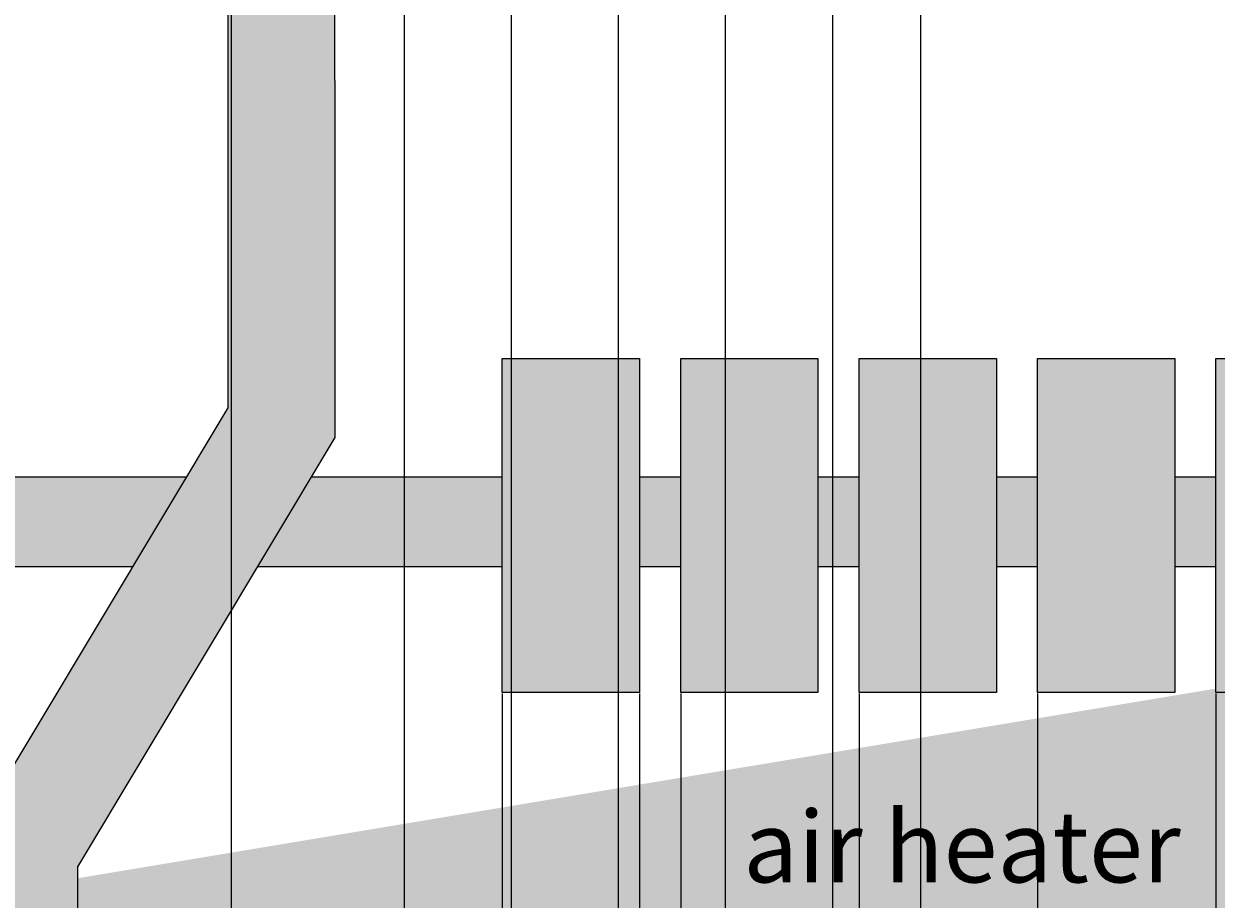
# Model space of a CAD drawing. Units: millimetres. Extents: x -22994 to 29398, y -19990 to 20176.
# Tile 109 of 135: x 99 to 166, y 124 to 174. Entities that reach past the tile are written whole.
import ezdxf

# ---------------------------------------------------------------- set-up
doc = ezdxf.new("R2010")
doc.units = ezdxf.units.MM
doc.header["$MEASUREMENT"] = 0
for name, color, linetype, lineweight in [('M-ANNO-TEXT', 7, 'Continuous', 25), ('M-DIMS', 2, 'Continuous', 18), ('M-EQPM', 7, 'Continuous', 25), ('M-EQPM-PATT', 7, 'Continuous', 18)]:
    doc.layers.add(name, color=color, linetype=linetype, lineweight=lineweight)
doc.styles.get("Standard").update_dxf_attribs({"font": 'arial.ttf'})
doc.dimstyles.get("Standard").update_dxf_attribs({"dimtxt": 0.18, "dimasz": 10000, "dimexe": 0.18, "dimexo": 0.0625, "dimgap": 0.09, "dimtad": 0, "dimtih": 1, "dimtoh": 1, "dimdec": 0, "dimzin": 0, "dimdsep": 46, "dimtxsty": 'Standard', "dimcen": 0.09, "dimadec": 0, "dimazin": 0, "dimtfac": 1, "dimtdec": 0, "dimtofl": 0, "dimtmove": 0, "dimatfit": 3, "dimfxl": 1, "dimtolj": 1, "dimtzin": 0, "dimlwd": 30, "dimarcsym": 0})

# ---------------------------------------------------------------- blocks, each defined once
blk = doc.blocks.new('*D2')
at = {"layer": 'Defpoints', "color": 0, "transparency": 16777216}
for p in [(6.677, 10.271), (290.852, 10.271), (290.852, -5.079)]:
    blk.add_point(p, dxfattribs=at)
at = {"layer": 'M-DIMS', "color": 0, "lineweight": -2, "transparency": 16777216}
for p, q in [((6.677, 10.209), (6.677, -5.259)), ((290.852, 10.209), (290.852, -5.259))]:
    blk.add_line(p, q, dxfattribs=at)
at = {"layer": 'M-DIMS', "color": 0, "lineweight": 30, "transparency": 16777216}
for p, q in [((-9993.323, -5.079), (-19993.323, -5.079)), ((10290.852, -5.079), (20290.852, -5.079))]:
    blk.add_line(p, q, dxfattribs=at)
at = {"layer": 'M-DIMS', "color": 0, "transparency": 16777216}
for points in [[(-9993.323, 1661.588), (-9993.323, -1671.745), (6.677, -5.079)], [(10290.852, 1661.588), (10290.852, -1671.745), (290.852, -5.079)]]:
    blk.add_solid(points, dxfattribs=at)
at = {"layer": 'M-DIMS', "color": 0, "transparency": 16777216, "insert": (148.765, -5.079), "char_height": 0.18, "attachment_point": 5}
blk.add_mtext('\\A1;284.2', dxfattribs=at)
blk = doc.blocks.new('*D3')
at = {"layer": 'Defpoints', "color": 0, "transparency": 16777216}
for p in [(110.265, 204.165), (110.265, 176.366), (95.833, 127.967)]:
    blk.add_point(p, dxfattribs=at)
at = {"layer": 'M-DIMS', "color": 0, "lineweight": 30, "transparency": 16777216}
for p, q in [((-9904.167, 204.165), (-19904.167, 204.165)), ((10110.265, 204.165), (20110.265, 204.165))]:
    blk.add_line(p, q, dxfattribs=at)
at = {"layer": 'M-DIMS', "color": 0, "lineweight": -2, "transparency": 16777216}
for p, q in [((95.833, 128.03), (95.833, 204.345)), ((110.265, 176.429), (110.265, 204.345))]:
    blk.add_line(p, q, dxfattribs=at)
at = {"layer": 'M-DIMS', "color": 0, "transparency": 16777216}
for points in [[(-9904.167, 1870.832), (-9904.167, -1462.501), (95.833, 204.165)], [(10110.265, 1870.832), (10110.265, -1462.501), (110.265, 204.165)]]:
    blk.add_solid(points, dxfattribs=at)
at = {"layer": 'M-DIMS', "color": 0, "transparency": 16777216, "insert": (103.049, 204.165), "char_height": 0.18, "attachment_point": 5}
blk.add_mtext('\\A1;14.432', dxfattribs=at)
blk = doc.blocks.new('*D4')
at = {"layer": 'Defpoints', "color": 0, "transparency": 16777216}
for p in [(116.265, 204.165), (110.265, 176.366), (116.265, 176.366)]:
    blk.add_point(p, dxfattribs=at)
at = {"layer": 'M-DIMS', "color": 0, "lineweight": 30, "transparency": 16777216}
for p, q in [((-9889.735, 204.165), (-19889.735, 204.165)), ((10116.265, 204.165), (20116.265, 204.165))]:
    blk.add_line(p, q, dxfattribs=at)
at = {"layer": 'M-DIMS', "color": 0, "lineweight": -2, "transparency": 16777216}
for p, q in [((110.265, 176.429), (110.265, 204.345)), ((116.265, 176.429), (116.265, 204.345))]:
    blk.add_line(p, q, dxfattribs=at)
at = {"layer": 'M-DIMS', "color": 0, "transparency": 16777216}
for points in [[(-9889.735, 1870.832), (-9889.735, -1462.501), (110.265, 204.165)], [(10116.265, 1870.832), (10116.265, -1462.501), (116.265, 204.165)]]:
    blk.add_solid(points, dxfattribs=at)
at = {"layer": 'M-DIMS', "color": 0, "transparency": 16777216, "insert": (113.265, 204.165), "char_height": 0.18, "attachment_point": 5}
blk.add_mtext('\\A1;6', dxfattribs=at)
blk = doc.blocks.new('*D5')
at = {"layer": 'Defpoints', "color": 0, "transparency": 16777216}
for p in [(181.265, 204.165), (116.265, 176.366), (181.265, 176.366)]:
    blk.add_point(p, dxfattribs=at)
at = {"layer": 'M-DIMS', "color": 0, "lineweight": 30, "transparency": 16777216}
for p, q in [((-9883.735, 204.165), (-19883.735, 204.165)), ((10181.265, 204.165), (20181.265, 204.165))]:
    blk.add_line(p, q, dxfattribs=at)
at = {"layer": 'M-DIMS', "color": 0, "lineweight": -2, "transparency": 16777216}
for p, q in [((116.265, 176.429), (116.265, 204.345)), ((181.265, 176.429), (181.265, 204.345))]:
    blk.add_line(p, q, dxfattribs=at)
at = {"layer": 'M-DIMS', "color": 0, "transparency": 16777216}
for points in [[(-9883.735, 1870.832), (-9883.735, -1462.501), (116.265, 204.165)], [(10181.265, 1870.832), (10181.265, -1462.501), (181.265, 204.165)]]:
    blk.add_solid(points, dxfattribs=at)
at = {"layer": 'M-DIMS', "color": 0, "transparency": 16777216, "insert": (148.765, 204.165), "char_height": 0.18, "attachment_point": 5}
blk.add_mtext('\\A1;65', dxfattribs=at)
blk = doc.blocks.new('*D6')
at = {"layer": 'Defpoints', "color": 0, "transparency": 16777216}
for p in [(187.265, 204.165), (181.265, 176.366), (187.265, 176.366)]:
    blk.add_point(p, dxfattribs=at)
at = {"layer": 'M-DIMS', "color": 0, "lineweight": 30, "transparency": 16777216}
for p, q in [((-9818.735, 204.165), (-19818.735, 204.165)), ((10187.265, 204.165), (20187.265, 204.165))]:
    blk.add_line(p, q, dxfattribs=at)
at = {"layer": 'M-DIMS', "color": 0, "lineweight": -2, "transparency": 16777216}
for p, q in [((181.265, 176.429), (181.265, 204.345)), ((187.265, 176.429), (187.265, 204.345))]:
    blk.add_line(p, q, dxfattribs=at)
at = {"layer": 'M-DIMS', "color": 0, "transparency": 16777216}
for points in [[(-9818.735, 1870.832), (-9818.735, -1462.501), (181.265, 204.165)], [(10187.265, 1870.832), (10187.265, -1462.501), (187.265, 204.165)]]:
    blk.add_solid(points, dxfattribs=at)
at = {"layer": 'M-DIMS', "color": 0, "transparency": 16777216, "insert": (184.265, 204.165), "char_height": 0.18, "attachment_point": 5}
blk.add_mtext('\\A1;6', dxfattribs=at)
blk = doc.blocks.new('*D7')
at = {"layer": 'Defpoints', "color": 0, "transparency": 16777216}
for p in [(201.697, 204.165), (187.265, 176.366), (201.697, 127.967)]:
    blk.add_point(p, dxfattribs=at)
at = {"layer": 'M-DIMS', "color": 0, "lineweight": 30, "transparency": 16777216}
for p, q in [((-9812.735, 204.165), (-19812.735, 204.165)), ((10201.697, 204.165), (20201.697, 204.165))]:
    blk.add_line(p, q, dxfattribs=at)
at = {"layer": 'M-DIMS', "color": 0, "lineweight": -2, "transparency": 16777216}
for p, q in [((187.265, 176.429), (187.265, 204.345)), ((201.697, 128.03), (201.697, 204.345))]:
    blk.add_line(p, q, dxfattribs=at)
at = {"layer": 'M-DIMS', "color": 0, "transparency": 16777216}
for points in [[(-9812.735, 1870.832), (-9812.735, -1462.501), (187.265, 204.165)], [(10201.697, 1870.832), (10201.697, -1462.501), (201.697, 204.165)]]:
    blk.add_solid(points, dxfattribs=at)
at = {"layer": 'M-DIMS', "color": 0, "transparency": 16777216, "insert": (194.481, 204.165), "char_height": 0.18, "attachment_point": 5}
blk.add_mtext('\\A1;14.432', dxfattribs=at)
blk = doc.blocks.new('*D8')
at = {"layer": 'Defpoints', "color": 0, "transparency": 16777216}
for p in [(227.648, 204.165), (227.648, 146.73), (201.697, 127.967)]:
    blk.add_point(p, dxfattribs=at)
at = {"layer": 'M-DIMS', "color": 0, "lineweight": 30, "transparency": 16777216}
for p, q in [((-9798.303, 204.165), (-19798.303, 204.165)), ((10227.648, 204.165), (20227.648, 204.165))]:
    blk.add_line(p, q, dxfattribs=at)
at = {"layer": 'M-DIMS', "color": 0, "lineweight": -2, "transparency": 16777216}
for p, q in [((201.697, 128.03), (201.697, 204.345)), ((227.648, 146.792), (227.648, 204.345))]:
    blk.add_line(p, q, dxfattribs=at)
at = {"layer": 'M-DIMS', "color": 0, "transparency": 16777216}
for points in [[(-9798.303, 1870.832), (-9798.303, -1462.501), (201.697, 204.165)], [(10227.648, 1870.832), (10227.648, -1462.501), (227.648, 204.165)]]:
    blk.add_solid(points, dxfattribs=at)
at = {"layer": 'M-DIMS', "color": 0, "transparency": 16777216, "insert": (214.673, 204.165), "char_height": 0.18, "attachment_point": 5}
blk.add_mtext('\\A1;25.95', dxfattribs=at)
blk = doc.blocks.new('*D9')
at = {"layer": 'Defpoints', "color": 0, "transparency": 16777216}
for p in [(187.265, 176.366), (306.202, 176.366), (290.852, 10.271)]:
    blk.add_point(p, dxfattribs=at)
at = {"layer": 'M-DIMS', "color": 0, "lineweight": 30, "transparency": 16777216}
for p, q in [((306.202, 10176.366), (306.202, 20176.366)), ((306.202, -9989.729), (306.202, -19989.729))]:
    blk.add_line(p, q, dxfattribs=at)
at = {"layer": 'M-DIMS', "color": 0, "lineweight": -2, "transparency": 16777216}
for p, q in [((187.327, 176.366), (306.382, 176.366)), ((290.915, 10.271), (306.382, 10.271))]:
    blk.add_line(p, q, dxfattribs=at)
at = {"layer": 'M-DIMS', "color": 0, "transparency": 16777216}
for points in [[(-1360.465, 10176.366), (1972.869, 10176.366), (306.202, 176.366)], [(-1360.465, -9989.729), (1972.869, -9989.729), (306.202, 10.271)]]:
    blk.add_solid(points, dxfattribs=at)
at = {"layer": 'M-DIMS', "color": 0, "transparency": 16777216, "insert": (306.202, 93.319), "char_height": 0.18, "attachment_point": 5}
blk.add_mtext('\\A1;166.1', dxfattribs=at)
blk = doc.blocks.new('*D10')
at = {"layer": 'Defpoints', "color": 0, "transparency": 16777216}
for p in [(125.65, 136.071), (133.346, 136.071), (133.346, -5.079)]:
    blk.add_point(p, dxfattribs=at)
at = {"layer": 'M-DIMS', "color": 0, "lineweight": -2, "transparency": 16777216}
for p, q in [((125.65, 136.009), (125.65, -5.259)), ((133.346, 136.009), (133.346, -5.259))]:
    blk.add_line(p, q, dxfattribs=at)
at = {"layer": 'M-DIMS', "color": 0, "lineweight": 30, "transparency": 16777216}
for p, q in [((-9874.35, -5.079), (-19874.35, -5.079)), ((10133.346, -5.079), (20133.346, -5.079))]:
    blk.add_line(p, q, dxfattribs=at)
at = {"layer": 'M-DIMS', "color": 0, "transparency": 16777216}
for points in [[(-9874.35, 1661.588), (-9874.35, -1671.745), (125.65, -5.079)], [(10133.346, 1661.588), (10133.346, -1671.745), (133.346, -5.079)]]:
    blk.add_solid(points, dxfattribs=at)
at = {"layer": 'M-DIMS', "color": 0, "transparency": 16777216, "insert": (129.498, -5.079), "char_height": 0.18, "attachment_point": 5}
blk.add_mtext('\\A1;7.696', dxfattribs=at)
blk = doc.blocks.new('*D11')
at = {"layer": 'Defpoints', "color": 0, "transparency": 16777216}
for p in [(133.346, 136.071), (135.65, 136.071), (135.65, -5.079)]:
    blk.add_point(p, dxfattribs=at)
at = {"layer": 'M-DIMS', "color": 0, "lineweight": -2, "transparency": 16777216}
for p, q in [((133.346, 136.009), (133.346, -5.259)), ((135.65, 136.009), (135.65, -5.259))]:
    blk.add_line(p, q, dxfattribs=at)
at = {"layer": 'M-DIMS', "color": 0, "lineweight": 30, "transparency": 16777216}
for p, q in [((-9866.654, -5.079), (-19866.654, -5.079)), ((10135.65, -5.079), (20135.65, -5.079))]:
    blk.add_line(p, q, dxfattribs=at)
at = {"layer": 'M-DIMS', "color": 0, "transparency": 16777216}
for points in [[(-9866.654, 1661.588), (-9866.654, -1671.745), (133.346, -5.079)], [(10135.65, 1661.588), (10135.65, -1671.745), (135.65, -5.079)]]:
    blk.add_solid(points, dxfattribs=at)
at = {"layer": 'M-DIMS', "color": 0, "transparency": 16777216, "insert": (134.498, -5.079), "char_height": 0.18, "attachment_point": 5}
blk.add_mtext('\\A1;2.304', dxfattribs=at)
blk = doc.blocks.new('*D12')
at = {"layer": 'Defpoints', "color": 0, "transparency": 16777216}
for p in [(135.65, 136.071), (145.65, 136.071), (145.65, -5.079)]:
    blk.add_point(p, dxfattribs=at)
at = {"layer": 'M-DIMS', "color": 0, "lineweight": -2, "transparency": 16777216}
for p, q in [((135.65, 136.009), (135.65, -5.259)), ((145.65, 136.009), (145.65, -5.259))]:
    blk.add_line(p, q, dxfattribs=at)
at = {"layer": 'M-DIMS', "color": 0, "lineweight": 30, "transparency": 16777216}
for p, q in [((-9864.35, -5.079), (-19864.35, -5.079)), ((10145.65, -5.079), (20145.65, -5.079))]:
    blk.add_line(p, q, dxfattribs=at)
at = {"layer": 'M-DIMS', "color": 0, "transparency": 16777216}
for points in [[(-9864.35, 1661.588), (-9864.35, -1671.745), (135.65, -5.079)], [(10145.65, 1661.588), (10145.65, -1671.745), (145.65, -5.079)]]:
    blk.add_solid(points, dxfattribs=at)
at = {"layer": 'M-DIMS', "color": 0, "transparency": 16777216, "insert": (140.65, -5.079), "char_height": 0.18, "attachment_point": 5}
blk.add_mtext('\\A1;10', dxfattribs=at)
blk = doc.blocks.new('*D13')
at = {"layer": 'Defpoints', "color": 0, "transparency": 16777216}
for p in [(145.65, 136.071), (155.65, 136.071), (155.65, -5.079)]:
    blk.add_point(p, dxfattribs=at)
at = {"layer": 'M-DIMS', "color": 0, "lineweight": -2, "transparency": 16777216}
for p, q in [((145.65, 136.009), (145.65, -5.259)), ((155.65, 136.009), (155.65, -5.259))]:
    blk.add_line(p, q, dxfattribs=at)
at = {"layer": 'M-DIMS', "color": 0, "lineweight": 30, "transparency": 16777216}
for p, q in [((-9854.35, -5.079), (-19854.35, -5.079)), ((10155.65, -5.079), (20155.65, -5.079))]:
    blk.add_line(p, q, dxfattribs=at)
at = {"layer": 'M-DIMS', "color": 0, "transparency": 16777216}
for points in [[(-9854.35, 1661.588), (-9854.35, -1671.745), (145.65, -5.079)], [(10155.65, 1661.588), (10155.65, -1671.745), (155.65, -5.079)]]:
    blk.add_solid(points, dxfattribs=at)
at = {"layer": 'M-DIMS', "color": 0, "transparency": 16777216, "insert": (150.65, -5.079), "char_height": 0.18, "attachment_point": 5}
blk.add_mtext('\\A1;10', dxfattribs=at)
blk = doc.blocks.new('*D14')
at = {"layer": 'Defpoints', "color": 0, "transparency": 16777216}
for p in [(155.65, 136.071), (165.65, 136.071), (165.65, -5.079)]:
    blk.add_point(p, dxfattribs=at)
at = {"layer": 'M-DIMS', "color": 0, "lineweight": -2, "transparency": 16777216}
for p, q in [((155.65, 136.009), (155.65, -5.259)), ((165.65, 136.009), (165.65, -5.259))]:
    blk.add_line(p, q, dxfattribs=at)
at = {"layer": 'M-DIMS', "color": 0, "lineweight": 30, "transparency": 16777216}
for p, q in [((-9844.35, -5.079), (-19844.35, -5.079)), ((10165.65, -5.079), (20165.65, -5.079))]:
    blk.add_line(p, q, dxfattribs=at)
at = {"layer": 'M-DIMS', "color": 0, "transparency": 16777216}
for points in [[(-9844.35, 1661.588), (-9844.35, -1671.745), (155.65, -5.079)], [(10165.65, 1661.588), (10165.65, -1671.745), (165.65, -5.079)]]:
    blk.add_solid(points, dxfattribs=at)
at = {"layer": 'M-DIMS', "color": 0, "transparency": 16777216, "insert": (160.65, -5.079), "char_height": 0.18, "attachment_point": 5}
blk.add_mtext('\\A1;10', dxfattribs=at)
blk = doc.blocks.new('*D15')
at = {"layer": 'Defpoints', "color": 0, "transparency": 16777216}
for p in [(173.346, 154.788), (173.346, 136.071), (306.202, 136.071)]:
    blk.add_point(p, dxfattribs=at)
at = {"layer": 'M-DIMS', "color": 0, "lineweight": 30, "transparency": 16777216}
for p, q in [((306.202, 10154.788), (306.202, 20154.788)), ((306.202, -9863.929), (306.202, -19863.929))]:
    blk.add_line(p, q, dxfattribs=at)
at = {"layer": 'M-DIMS', "color": 0, "lineweight": -2, "transparency": 16777216}
for p, q in [((173.408, 154.788), (306.382, 154.788)), ((173.408, 136.071), (306.382, 136.071))]:
    blk.add_line(p, q, dxfattribs=at)
at = {"layer": 'M-DIMS', "color": 0, "transparency": 16777216}
for points in [[(-1360.465, 10154.788), (1972.869, 10154.788), (306.202, 154.788)], [(-1360.465, -9863.929), (1972.869, -9863.929), (306.202, 136.071)]]:
    blk.add_solid(points, dxfattribs=at)
at = {"layer": 'M-DIMS', "color": 0, "transparency": 16777216, "insert": (306.202, 145.43), "char_height": 0.18, "attachment_point": 5}
blk.add_mtext('\\A1;18.717', dxfattribs=at)
blk = doc.blocks.new('*D16')
at = {"layer": 'Defpoints', "color": 0, "transparency": 16777216}
for p in [(120.17, 204.165), (110.466, 48.035), (120.17, 48.035)]:
    blk.add_point(p, dxfattribs=at)
at = {"layer": 'M-DIMS', "color": 0, "lineweight": 30, "transparency": 16777216}
for p, q in [((-9889.534, 204.165), (-19889.534, 204.165)), ((10120.17, 204.165), (20120.17, 204.165))]:
    blk.add_line(p, q, dxfattribs=at)
at = {"layer": 'M-DIMS', "color": 0, "lineweight": -2, "transparency": 16777216}
for p, q in [((110.466, 48.097), (110.466, 204.345)), ((120.17, 48.097), (120.17, 204.345))]:
    blk.add_line(p, q, dxfattribs=at)
at = {"layer": 'M-DIMS', "color": 0, "transparency": 16777216}
for points in [[(-9889.534, 1870.832), (-9889.534, -1462.501), (110.466, 204.165)], [(10120.17, 1870.832), (10120.17, -1462.501), (120.17, 204.165)]]:
    blk.add_solid(points, dxfattribs=at)
at = {"layer": 'M-DIMS', "color": 0, "transparency": 16777216, "insert": (115.318, 204.165), "char_height": 0.18, "attachment_point": 5}
blk.add_mtext('\\A1;9.704', dxfattribs=at)
blk = doc.blocks.new('*D17')
at = {"layer": 'Defpoints', "color": 0, "transparency": 16777216}
for p in [(126.17, 204.165), (120.17, 48.035), (126.17, 48.035)]:
    blk.add_point(p, dxfattribs=at)
at = {"layer": 'M-DIMS', "color": 0, "lineweight": 30, "transparency": 16777216}
for p, q in [((-9879.83, 204.165), (-19879.83, 204.165)), ((10126.17, 204.165), (20126.17, 204.165))]:
    blk.add_line(p, q, dxfattribs=at)
at = {"layer": 'M-DIMS', "color": 0, "lineweight": -2, "transparency": 16777216}
for p, q in [((120.17, 48.097), (120.17, 204.345)), ((126.17, 48.097), (126.17, 204.345))]:
    blk.add_line(p, q, dxfattribs=at)
at = {"layer": 'M-DIMS', "color": 0, "transparency": 16777216}
for points in [[(-9879.83, 1870.832), (-9879.83, -1462.501), (120.17, 204.165)], [(10126.17, 1870.832), (10126.17, -1462.501), (126.17, 204.165)]]:
    blk.add_solid(points, dxfattribs=at)
at = {"layer": 'M-DIMS', "color": 0, "transparency": 16777216, "insert": (123.17, 204.165), "char_height": 0.18, "attachment_point": 5}
blk.add_mtext('\\A1;6', dxfattribs=at)
blk = doc.blocks.new('*D18')
at = {"layer": 'Defpoints', "color": 0, "transparency": 16777216}
for p in [(132.17, 204.165), (126.17, 48.035), (132.17, 48.035)]:
    blk.add_point(p, dxfattribs=at)
at = {"layer": 'M-DIMS', "color": 0, "lineweight": 30, "transparency": 16777216}
for p, q in [((-9873.83, 204.165), (-19873.83, 204.165)), ((10132.17, 204.165), (20132.17, 204.165))]:
    blk.add_line(p, q, dxfattribs=at)
at = {"layer": 'M-DIMS', "color": 0, "lineweight": -2, "transparency": 16777216}
for p, q in [((126.17, 48.097), (126.17, 204.345)), ((132.17, 48.097), (132.17, 204.345))]:
    blk.add_line(p, q, dxfattribs=at)
at = {"layer": 'M-DIMS', "color": 0, "transparency": 16777216}
for points in [[(-9873.83, 1870.832), (-9873.83, -1462.501), (126.17, 204.165)], [(10132.17, 1870.832), (10132.17, -1462.501), (132.17, 204.165)]]:
    blk.add_solid(points, dxfattribs=at)
at = {"layer": 'M-DIMS', "color": 0, "transparency": 16777216, "insert": (129.17, 204.165), "char_height": 0.18, "attachment_point": 5}
blk.add_mtext('\\A1;6', dxfattribs=at)
blk = doc.blocks.new('*D19')
at = {"layer": 'Defpoints', "color": 0, "transparency": 16777216}
for p in [(138.17, 204.165), (132.17, 48.035), (138.17, 48.035)]:
    blk.add_point(p, dxfattribs=at)
at = {"layer": 'M-DIMS', "color": 0, "lineweight": 30, "transparency": 16777216}
for p, q in [((-9867.83, 204.165), (-19867.83, 204.165)), ((10138.17, 204.165), (20138.17, 204.165))]:
    blk.add_line(p, q, dxfattribs=at)
at = {"layer": 'M-DIMS', "color": 0, "lineweight": -2, "transparency": 16777216}
for p, q in [((132.17, 48.097), (132.17, 204.345)), ((138.17, 48.097), (138.17, 204.345))]:
    blk.add_line(p, q, dxfattribs=at)
at = {"layer": 'M-DIMS', "color": 0, "transparency": 16777216}
for points in [[(-9867.83, 1870.832), (-9867.83, -1462.501), (132.17, 204.165)], [(10138.17, 1870.832), (10138.17, -1462.501), (138.17, 204.165)]]:
    blk.add_solid(points, dxfattribs=at)
at = {"layer": 'M-DIMS', "color": 0, "transparency": 16777216, "insert": (135.17, 204.165), "char_height": 0.18, "attachment_point": 5}
blk.add_mtext('\\A1;6', dxfattribs=at)
blk = doc.blocks.new('*D20')
at = {"layer": 'Defpoints', "color": 0, "transparency": 16777216}
for p in [(144.17, 204.165), (138.17, 48.035), (144.17, 48.035)]:
    blk.add_point(p, dxfattribs=at)
at = {"layer": 'M-DIMS', "color": 0, "lineweight": 30, "transparency": 16777216}
for p, q in [((-9861.83, 204.165), (-19861.83, 204.165)), ((10144.17, 204.165), (20144.17, 204.165))]:
    blk.add_line(p, q, dxfattribs=at)
at = {"layer": 'M-DIMS', "color": 0, "lineweight": -2, "transparency": 16777216}
for p, q in [((138.17, 48.097), (138.17, 204.345)), ((144.17, 48.097), (144.17, 204.345))]:
    blk.add_line(p, q, dxfattribs=at)
at = {"layer": 'M-DIMS', "color": 0, "transparency": 16777216}
for points in [[(-9861.83, 1870.832), (-9861.83, -1462.501), (138.17, 204.165)], [(10144.17, 1870.832), (10144.17, -1462.501), (144.17, 204.165)]]:
    blk.add_solid(points, dxfattribs=at)
at = {"layer": 'M-DIMS', "color": 0, "transparency": 16777216, "insert": (141.17, 204.165), "char_height": 0.18, "attachment_point": 5}
blk.add_mtext('\\A1;6', dxfattribs=at)
blk = doc.blocks.new('*D21')
at = {"layer": 'Defpoints', "color": 0, "transparency": 16777216}
for p in [(149.116, 204.165), (144.17, 48.035), (149.116, 48.035)]:
    blk.add_point(p, dxfattribs=at)
at = {"layer": 'M-DIMS', "color": 0, "lineweight": 30, "transparency": 16777216}
for p, q in [((-9855.83, 204.165), (-19855.83, 204.165)), ((10149.116, 204.165), (20149.116, 204.165))]:
    blk.add_line(p, q, dxfattribs=at)
at = {"layer": 'M-DIMS', "color": 0, "lineweight": -2, "transparency": 16777216}
for p, q in [((144.17, 48.097), (144.17, 204.345)), ((149.116, 48.097), (149.116, 204.345))]:
    blk.add_line(p, q, dxfattribs=at)
at = {"layer": 'M-DIMS', "color": 0, "transparency": 16777216}
for points in [[(-9855.83, 1870.832), (-9855.83, -1462.501), (144.17, 204.165)], [(10149.116, 1870.832), (10149.116, -1462.501), (149.116, 204.165)]]:
    blk.add_solid(points, dxfattribs=at)
at = {"layer": 'M-DIMS', "color": 0, "transparency": 16777216, "insert": (146.643, 204.165), "char_height": 0.18, "attachment_point": 5}
blk.add_mtext('\\A1;4.945', dxfattribs=at)
blk = doc.blocks.new('*D22')
at = {"layer": 'Defpoints', "color": 0, "transparency": 16777216}
for p in [(149.116, 30.99), (155.116, 30.99), (155.116, -5.079)]:
    blk.add_point(p, dxfattribs=at)
at = {"layer": 'M-DIMS', "color": 0, "lineweight": -2, "transparency": 16777216}
for p, q in [((149.116, 30.927), (149.116, -5.259)), ((155.116, 30.927), (155.116, -5.259))]:
    blk.add_line(p, q, dxfattribs=at)
at = {"layer": 'M-DIMS', "color": 0, "lineweight": 30, "transparency": 16777216}
for p, q in [((-9850.884, -5.079), (-19850.884, -5.079)), ((10155.116, -5.079), (20155.116, -5.079))]:
    blk.add_line(p, q, dxfattribs=at)
at = {"layer": 'M-DIMS', "color": 0, "transparency": 16777216}
for points in [[(-9850.884, 1661.588), (-9850.884, -1671.745), (149.116, -5.079)], [(10155.116, 1661.588), (10155.116, -1671.745), (155.116, -5.079)]]:
    blk.add_solid(points, dxfattribs=at)
at = {"layer": 'M-DIMS', "color": 0, "transparency": 16777216, "insert": (152.116, -5.079), "char_height": 0.18, "attachment_point": 5}
blk.add_mtext('\\A1;6', dxfattribs=at)
blk = doc.blocks.new('*D23')
at = {"layer": 'Defpoints', "color": 0, "transparency": 16777216}
for p in [(155.116, 30.99), (161.116, 30.99), (161.116, -5.079)]:
    blk.add_point(p, dxfattribs=at)
at = {"layer": 'M-DIMS', "color": 0, "lineweight": -2, "transparency": 16777216}
for p, q in [((155.116, 30.927), (155.116, -5.259)), ((161.116, 30.927), (161.116, -5.259))]:
    blk.add_line(p, q, dxfattribs=at)
at = {"layer": 'M-DIMS', "color": 0, "lineweight": 30, "transparency": 16777216}
for p, q in [((-9844.884, -5.079), (-19844.884, -5.079)), ((10161.116, -5.079), (20161.116, -5.079))]:
    blk.add_line(p, q, dxfattribs=at)
at = {"layer": 'M-DIMS', "color": 0, "transparency": 16777216}
for points in [[(-9844.884, 1661.588), (-9844.884, -1671.745), (155.116, -5.079)], [(10161.116, 1661.588), (10161.116, -1671.745), (161.116, -5.079)]]:
    blk.add_solid(points, dxfattribs=at)
at = {"layer": 'M-DIMS', "color": 0, "transparency": 16777216, "insert": (158.116, -5.079), "char_height": 0.18, "attachment_point": 5}
blk.add_mtext('\\A1;6', dxfattribs=at)
blk = doc.blocks.new('*D24')
at = {"layer": 'Defpoints', "color": 0, "transparency": 16777216}
for p in [(161.116, 30.99), (166.439, 30.99), (166.439, -5.079)]:
    blk.add_point(p, dxfattribs=at)
at = {"layer": 'M-DIMS', "color": 0, "lineweight": -2, "transparency": 16777216}
for p, q in [((161.116, 30.927), (161.116, -5.259)), ((166.439, 30.927), (166.439, -5.259))]:
    blk.add_line(p, q, dxfattribs=at)
at = {"layer": 'M-DIMS', "color": 0, "lineweight": 30, "transparency": 16777216}
for p, q in [((-9838.884, -5.079), (-19838.884, -5.079)), ((10166.439, -5.079), (20166.439, -5.079))]:
    blk.add_line(p, q, dxfattribs=at)
at = {"layer": 'M-DIMS', "color": 0, "transparency": 16777216}
for points in [[(-9838.884, 1661.588), (-9838.884, -1671.745), (161.116, -5.079)], [(10166.439, 1661.588), (10166.439, -1671.745), (166.439, -5.079)]]:
    blk.add_solid(points, dxfattribs=at)
at = {"layer": 'M-DIMS', "color": 0, "transparency": 16777216, "insert": (163.777, -5.079), "char_height": 0.18, "attachment_point": 5}
blk.add_mtext('\\A1;5.323', dxfattribs=at)
blk = doc.blocks.new('*D25')
at = {"layer": 'Defpoints', "color": 0, "transparency": 16777216}
for p in [(166.439, 30.99), (172.439, 30.99), (172.439, -5.079)]:
    blk.add_point(p, dxfattribs=at)
at = {"layer": 'M-DIMS', "color": 0, "lineweight": -2, "transparency": 16777216}
for p, q in [((166.439, 30.927), (166.439, -5.259)), ((172.439, 30.927), (172.439, -5.259))]:
    blk.add_line(p, q, dxfattribs=at)
at = {"layer": 'M-DIMS', "color": 0, "lineweight": 30, "transparency": 16777216}
for p, q in [((-9833.561, -5.079), (-19833.561, -5.079)), ((10172.439, -5.079), (20172.439, -5.079))]:
    blk.add_line(p, q, dxfattribs=at)
at = {"layer": 'M-DIMS', "color": 0, "transparency": 16777216}
for points in [[(-9833.561, 1661.588), (-9833.561, -1671.745), (166.439, -5.079)], [(10172.439, 1661.588), (10172.439, -1671.745), (172.439, -5.079)]]:
    blk.add_solid(points, dxfattribs=at)
at = {"layer": 'M-DIMS', "color": 0, "transparency": 16777216, "insert": (169.439, -5.079), "char_height": 0.18, "attachment_point": 5}
blk.add_mtext('\\A1;6', dxfattribs=at)
blk = doc.blocks.new('*D26')
at = {"layer": 'Defpoints', "color": 0, "transparency": 16777216}
for p in [(172.439, 30.99), (178.439, 30.99), (178.439, -5.079)]:
    blk.add_point(p, dxfattribs=at)
at = {"layer": 'M-DIMS', "color": 0, "lineweight": -2, "transparency": 16777216}
for p, q in [((172.439, 30.927), (172.439, -5.259)), ((178.439, 30.927), (178.439, -5.259))]:
    blk.add_line(p, q, dxfattribs=at)
at = {"layer": 'M-DIMS', "color": 0, "lineweight": 30, "transparency": 16777216}
for p, q in [((-9827.561, -5.079), (-19827.561, -5.079)), ((10178.439, -5.079), (20178.439, -5.079))]:
    blk.add_line(p, q, dxfattribs=at)
at = {"layer": 'M-DIMS', "color": 0, "transparency": 16777216}
for points in [[(-9827.561, 1661.588), (-9827.561, -1671.745), (172.439, -5.079)], [(10178.439, 1661.588), (10178.439, -1671.745), (178.439, -5.079)]]:
    blk.add_solid(points, dxfattribs=at)
at = {"layer": 'M-DIMS', "color": 0, "transparency": 16777216, "insert": (175.439, -5.079), "char_height": 0.18, "attachment_point": 5}
blk.add_mtext('\\A1;6', dxfattribs=at)
blk = doc.blocks.new('*D27')
at = {"layer": 'Defpoints', "color": 0, "transparency": 16777216}
for p in [(178.439, 30.99), (188.117, 30.99), (188.117, -5.079)]:
    blk.add_point(p, dxfattribs=at)
at = {"layer": 'M-DIMS', "color": 0, "lineweight": -2, "transparency": 16777216}
for p, q in [((178.439, 30.927), (178.439, -5.259)), ((188.117, 30.927), (188.117, -5.259))]:
    blk.add_line(p, q, dxfattribs=at)
at = {"layer": 'M-DIMS', "color": 0, "lineweight": 30, "transparency": 16777216}
for p, q in [((-9821.561, -5.079), (-19821.561, -5.079)), ((10188.117, -5.079), (20188.117, -5.079))]:
    blk.add_line(p, q, dxfattribs=at)
at = {"layer": 'M-DIMS', "color": 0, "transparency": 16777216}
for points in [[(-9821.561, 1661.588), (-9821.561, -1671.745), (178.439, -5.079)], [(10188.117, 1661.588), (10188.117, -1671.745), (188.117, -5.079)]]:
    blk.add_solid(points, dxfattribs=at)
at = {"layer": 'M-DIMS', "color": 0, "transparency": 16777216, "insert": (183.278, -5.079), "char_height": 0.18, "attachment_point": 5}
blk.add_mtext('\\A1;9.679', dxfattribs=at)
blk = doc.blocks.new('*D28')
at = {"layer": 'Defpoints', "color": 0, "transparency": 16777216}
for p in [(188.117, 48.035), (306.202, 48.035), (188.117, 30.99)]:
    blk.add_point(p, dxfattribs=at)
at = {"layer": 'M-DIMS', "color": 0, "lineweight": 30, "transparency": 16777216}
for p, q in [((306.202, 10048.035), (306.202, 20048.035)), ((306.202, -9969.01), (306.202, -19969.01))]:
    blk.add_line(p, q, dxfattribs=at)
at = {"layer": 'M-DIMS', "color": 0, "lineweight": -2, "transparency": 16777216}
for p, q in [((188.18, 48.035), (306.382, 48.035)), ((188.18, 30.99), (306.382, 30.99))]:
    blk.add_line(p, q, dxfattribs=at)
at = {"layer": 'M-DIMS', "color": 0, "transparency": 16777216}
for points in [[(-1360.465, 10048.035), (1972.869, 10048.035), (306.202, 48.035)], [(-1360.465, -9969.01), (1972.869, -9969.01), (306.202, 30.99)]]:
    blk.add_solid(points, dxfattribs=at)
at = {"layer": 'M-DIMS', "color": 0, "transparency": 16777216, "insert": (306.202, 39.512), "char_height": 0.18, "attachment_point": 5}
blk.add_mtext('\\A1;17.045', dxfattribs=at)
blk = doc.blocks.new('*D29')
at = {"layer": 'Defpoints', "color": 0, "transparency": 16777216}
for p in [(36.801, 80.045), (64.03, 80.045)]:
    blk.add_point(p, dxfattribs=at)
at = {"layer": 'M-DIMS', "color": 0, "lineweight": -2, "transparency": 16777216}
for p, q in [((50.325, 80.045), (50.505, 80.045)), ((50.415, 79.955), (50.415, 80.135))]:
    blk.add_line(p, q, dxfattribs=at)
at = {"layer": 'M-DIMS', "color": 0, "lineweight": 30, "transparency": 16777216}
blk.add_line((20064.03, 80.03), (10064.03, 80.038), dxfattribs=at)
at = {"layer": 'M-DIMS', "color": 0, "transparency": 16777216}
blk.add_solid([(10064.031, 1746.704), (10064.028, -1586.629), (64.03, 80.045)], dxfattribs=at)
at = {"layer": 'M-DIMS', "color": 0, "transparency": 16777216, "insert": (20064.521, 80.03), "char_height": 0.18, "attachment_point": 5}
blk.add_mtext('\\A1;∅27.23', dxfattribs=at)
blk = doc.blocks.new('*D36')
at = {"layer": 'Defpoints', "color": 0, "transparency": 16777216}
for p in [(46.39, 31.303), (46.387, 26.593)]:
    blk.add_point(p, dxfattribs=at)
at = {"layer": 'M-DIMS', "color": 0, "lineweight": 30, "transparency": 16777216}
for p, q in [((57.15, 20031.301), (51.77, 10031.302)), ((10057.15, 20031.301), (57.15, 20031.301))]:
    blk.add_line(p, q, dxfattribs=at)
at = {"layer": 'M-DIMS', "color": 0, "lineweight": -2, "transparency": 16777216}
for p, q in [((46.299, 28.948), (46.479, 28.948)), ((46.389, 28.858), (46.389, 29.038))]:
    blk.add_line(p, q, dxfattribs=at)
at = {"layer": 'M-DIMS', "color": 0, "transparency": 16777216}
blk.add_solid([(-1614.896, 10032.199), (1718.436, 10030.405), (46.39, 31.303)], dxfattribs=at)
at = {"layer": 'M-DIMS', "color": 0, "transparency": 16777216, "insert": (10057.554, 20031.301), "char_height": 0.18, "attachment_point": 5}
blk.add_mtext('\\A1;∅4.71', dxfattribs=at)
blk = doc.blocks.new('*D37')
at = {"layer": 'Defpoints', "color": 0, "transparency": 16777216}
for p in [(54.834, 118.615), (59.494, 118.614)]:
    blk.add_point(p, dxfattribs=at)
at = {"layer": 'M-DIMS', "color": 0, "lineweight": -2, "transparency": 16777216}
for p, q in [((57.074, 118.614), (57.254, 118.614)), ((57.164, 118.524), (57.164, 118.704))]:
    blk.add_line(p, q, dxfattribs=at)
at = {"layer": 'M-DIMS', "color": 0, "lineweight": 30, "transparency": 16777216}
blk.add_line((20059.493, 116.253), (10059.494, 117.434), dxfattribs=at)
at = {"layer": 'M-DIMS', "color": 0, "transparency": 16777216}
blk.add_solid([(10059.69, 1784.1), (10059.297, -1549.233), (59.494, 118.614)], dxfattribs=at)
at = {"layer": 'M-DIMS', "color": 0, "transparency": 16777216, "insert": (20059.985, 116.253), "char_height": 0.18, "attachment_point": 5}
blk.add_mtext('\\A1;∅4.659', dxfattribs=at)

msp = doc.modelspace()

# ---------------------------------------------------------------- hatches: boundary and pattern name
at = {"layer": 'M-EQPM-PATT'}
h = msp.add_hatch(color=256, dxfattribs=at)
h.set_gradient(color1=(205, 32, 39), color2=(205, 32, 39), tint=1)
h.paths.add_polyline_path([(116.2647, 150.3662), (116.2647, 170.3662), (116.2647, 176.3662), (110.2647, 176.3662), (110.2647, 152.0276), (95.8327, 127.967), (95.8327, 16.6063), (201.6967, 16.6063), (201.6967, 127.967), (187.2647, 152.0276), (187.2647, 176.3662), (181.2647, 176.3662), (181.2647, 170.3662), (181.2647, 150.3662), (195.6967, 126.3055), (195.6967, 22.6063), (101.8327, 22.6063), (101.8327, 126.3055)])
h.paths.add_polyline_path([(185.2208, 88.6347), (101.8327, 88.6347), (101.8327, 87.6347), (182.8066, 87.6347), (178.7313, 83.5594), (195.6967, 83.5594), (195.6967, 84.5594), (181.1455, 84.5594)], flags=17)
h.paths.add_polyline_path([(95.8327, 88.6347), (60.9779, 88.6347, -0.0228552), (61.7178, 87.6347), (95.8327, 87.6347)])
h.paths.add_polyline_path([(215.6212, 86.5189), (215.6212, 80.5999), (220.5095, 83.5594)])
h.paths.add_polyline_path([(215.6212, 84.5594), (201.6967, 84.5594), (201.6967, 83.5594), (215.6212, 83.5594)])
h.paths.add_polyline_path([(225.3978, 86.5189), (220.5095, 83.5594), (225.3978, 80.5999)])
h.paths.add_polyline_path([(231.6256, 84.5594), (225.3978, 84.5594), (225.3978, 83.5594), (231.6256, 83.5594)])
h = msp.add_hatch(color=256, dxfattribs=at)
h.set_gradient(color1=(128, 128, 128), color2=(128, 128, 128), tint=1)
h.paths.add_polyline_path([(88.0003, 148.1301), (88.0003, 143.1301), (104.9278, 143.1301), (107.9269, 148.1301)])
h.paths.add_polyline_path([(189.6025, 148.1301), (192.6016, 143.1301), (216.9016, 143.1301, -0.0809736), (216.3148, 146.7296, -0.0309822), (216.4017, 148.1301)])
h.paths.add_polyline_path([(229.9653, 167.6546), (245.0476, 167.6546), (245.0476, 172.6546), (224.9653, 172.6546), (224.9653, 157.741, -0.1116822), (229.9653, 157.8239)])
h.paths.add_polyline_path([(36.3887, 21.6644), (36.3887, 16.6063), (56.3887, 16.6063), (56.3887, 21.6644)])
h = msp.add_hatch(color=256, dxfattribs=at)
h.set_gradient(color1=(147, 39, 143), color2=(147, 39, 143), tint=1)
h.paths.add_polyline_path([(125.6498, 136.0713), (133.3459, 136.0713), (133.3459, 154.788), (125.6498, 154.788)])
h.paths.add_polyline_path([(135.6498, 136.0713), (143.3459, 136.0713), (143.3459, 154.788), (135.6498, 154.788)])
h.paths.add_polyline_path([(145.6498, 136.0713), (153.3459, 136.0713), (153.3459, 154.788), (145.6498, 154.788)])
h.paths.add_polyline_path([(155.6498, 136.0713), (163.3459, 136.0713), (163.3459, 154.788), (155.6498, 154.788)])
h.paths.add_polyline_path([(165.6498, 136.0713), (173.3459, 136.0713), (173.3459, 154.788), (165.6498, 154.788)])
h = msp.add_hatch(color=256, dxfattribs=at)
h.set_gradient(color1=(19, 155, 72), color2=(19, 155, 72), tint=1)
h.paths.add_polyline_path([(114.9234, 148.1301), (111.9243, 143.1301), (125.6498, 143.1301), (125.6498, 148.1301)])
h.paths.add_polyline_path([(173.3459, 148.1301), (173.3459, 143.1301), (185.605, 143.1301), (182.6059, 148.1301)])
h.paths.add_polyline_path([(135.6498, 148.1301), (133.3459, 148.1301), (133.3459, 143.1301), (135.6498, 143.1301)])
h.paths.add_polyline_path([(143.3459, 143.1301), (145.6498, 143.1301), (145.6498, 148.1301), (143.3459, 148.1301)])
h.paths.add_polyline_path([(153.3459, 143.1301), (155.6498, 143.1301), (155.6498, 148.1301), (153.3459, 148.1301)])
h.paths.add_polyline_path([(165.6498, 148.1301), (163.3459, 148.1301), (163.3459, 143.1301), (165.6498, 143.1301)])

# ---------------------------------------------------------------- linework, layer by layer
at = {"layer": 'M-EQPM'}
for p, q in [((116.2647, 170.3662), (116.2647, 176.3662)), ((107.9269, 148.1301), (88.0003, 148.1301)), ((125.6498, 148.1301), (114.9234, 148.1301)), ((135.6498, 148.1301), (133.3459, 148.1301)), ((145.6498, 148.1301), (143.3459, 148.1301)), ((155.6498, 148.1301), (153.3459, 148.1301)), ((165.6498, 148.1301), (163.3459, 148.1301)), ((88.0003, 143.1301), (104.9278, 143.1301)), ((111.9243, 143.1301), (125.6498, 143.1301)), ((133.3459, 143.1301), (135.6498, 143.1301)), ((143.3459, 143.1301), (145.6498, 143.1301)), ((153.3459, 143.1301), (155.6498, 143.1301)), ((163.3459, 143.1301), (165.6498, 143.1301))]:
    msp.add_line(p, q, dxfattribs=at)
for points in [[(110.2647, 176.3662), (110.2647, 152.0276), (95.8327, 127.967), (95.8327, 16.6063), (201.6967, 16.6063), (201.6967, 127.967), (187.2647, 152.0276), (187.2647, 176.3662)], [(125.6498, 154.788), (133.3459, 154.788), (133.3459, 136.0713), (125.6498, 136.0713)], [(135.6498, 154.788), (143.3459, 154.788), (143.3459, 136.0713), (135.6498, 136.0713)], [(145.6498, 154.788), (153.3459, 154.788), (153.3459, 136.0713), (145.6498, 136.0713)], [(155.6498, 154.788), (163.3459, 154.788), (163.3459, 136.0713), (155.6498, 136.0713)], [(165.6498, 154.788), (173.3459, 154.788), (173.3459, 136.0713), (165.6498, 136.0713)]]:
    msp.add_lwpolyline(points, close=True, dxfattribs=at)
msp.add_lwpolyline([(116.2647, 170.3662), (116.2647, 150.3662), (101.8327, 126.3055), (101.8327, 22.6063), (195.6967, 22.6063), (195.6967, 126.3055), (181.2647, 150.3662), (181.2647, 170.3662)], dxfattribs=at)

# ---------------------------------------------------------------- texts
at = {"layer": 'M-ANNO-TEXT', "insert": (139.1568, 129.4339), "char_height": 4, "attachment_point": 1}
msp.add_mtext_dynamic_manual_height_columns('air heater', width=37.883315, gutter_width=1, heights=[0], dxfattribs=at)

# ---------------------------------------------------------------- dimensions: what is measured, and where the dimension line sits
at = {"layer": 'M-DIMS'}
for base, p1, p2, override, picture, middle in [((306.202, 176.3662), (290.852, 10.2713), (187.2647, 176.3662), {"dimdec": 1, "dimlfac": 1, "dimrnd": 0, "dimzin": 0, "dimdsep": 46, "dimlunit": 2}, '*D9', (306.202, 93.3187)), ((306.202, 136.0713), (173.3459, 154.788), (173.3459, 136.0713), {"dimdec": 3, "dimlfac": 1, "dimrnd": 0, "dimzin": 0, "dimdsep": 46, "dimlunit": 2}, '*D15', (306.202, 145.4297)), ((306.202, 48.0349), (188.1175, 30.9895), (188.1175, 48.0349), {"dimdec": 3, "dimlfac": 1, "dimrnd": 0, "dimzin": 0, "dimdsep": 46, "dimlunit": 2}, '*D28', (306.202, 39.5122))]:
    dim = msp.add_linear_dim(base=base, p1=p1, p2=p2, angle=90, dimstyle='Standard', override=override, dxfattribs=at)
    dim.commit()
    dim.dimension.update_dxf_attribs({"geometry": picture, "text_midpoint": middle})
dim = msp.add_diameter_dim_2p(p1=(46.3875, 26.5934), p2=(46.39, 31.3035), dimstyle='Standard', override={"dimdec": 2, "dimlfac": 1, "dimrnd": 0, "dimzin": 0, "dimdsep": 46, "dimlunit": 2}, dxfattribs=at)
dim.commit()
dim.dimension.update_dxf_attribs({"geometry": '*D36', "text_midpoint": (10057.5542, 20031.3006), "dimtype": 163})
for base, p1, p2, override, picture, middle in [((110.2647, 204.1654), (95.8327, 127.967), (110.2647, 176.3662), {"dimdec": 3, "dimlfac": 1, "dimrnd": 0, "dimzin": 0, "dimdsep": 46, "dimlunit": 2}, '*D3', (103.0487, 204.1654)), ((116.2647, 204.1654), (110.2647, 176.3662), (116.2647, 176.3662), {"dimdec": 0, "dimlfac": 1, "dimrnd": 0, "dimzin": 0, "dimdsep": 46, "dimlunit": 2}, '*D4', (113.2647, 204.1654)), ((120.1702, 204.1654), (110.4658, 48.0349), (120.1702, 48.0349), {"dimdec": 3, "dimlfac": 1, "dimrnd": 0, "dimzin": 0, "dimdsep": 46, "dimlunit": 2}, '*D16', (115.318, 204.1654)), ((181.2647, 204.1654), (116.2647, 176.3662), (181.2647, 176.3662), {"dimdec": 0, "dimlfac": 1, "dimrnd": 0, "dimzin": 0, "dimdsep": 46, "dimlunit": 2}, '*D5', (148.7647, 204.1654)), ((126.1702, 204.1654), (120.1702, 48.0349), (126.1702, 48.0349), {"dimdec": 0, "dimlfac": 1, "dimrnd": 0, "dimzin": 0, "dimdsep": 46, "dimlunit": 2}, '*D17', (123.1702, 204.1654)), ((132.1702, 204.1654), (126.1702, 48.0349), (132.1702, 48.0349), {"dimdec": 0, "dimlfac": 1, "dimrnd": 0, "dimzin": 0, "dimdsep": 46, "dimlunit": 2}, '*D18', (129.1702, 204.1654)), ((138.1702, 204.1654), (132.1702, 48.0349), (138.1702, 48.0349), {"dimdec": 0, "dimlfac": 1, "dimrnd": 0, "dimzin": 0, "dimdsep": 46, "dimlunit": 2}, '*D19', (135.1702, 204.1654)), ((144.1702, 204.1654), (138.1702, 48.0349), (144.1702, 48.0349), {"dimdec": 0, "dimlfac": 1, "dimrnd": 0, "dimzin": 0, "dimdsep": 46, "dimlunit": 2}, '*D20', (141.1702, 204.1654)), ((149.11567, 204.16539), (144.17023, 48.03494), (149.11567, 48.03494), {"dimdec": 3, "dimlfac": 1, "dimrnd": 0, "dimzin": 0, "dimdsep": 46, "dimlunit": 2}, '*D21', (146.64295, 204.16539)), ((187.2647, 204.1654), (181.2647, 176.3662), (187.2647, 176.3662), {"dimdec": 0, "dimlfac": 1, "dimrnd": 0, "dimzin": 0, "dimdsep": 46, "dimlunit": 2}, '*D6', (184.2647, 204.1654)), ((201.6967, 204.1654), (187.2647, 176.3662), (201.6967, 127.967), {"dimdec": 3, "dimlfac": 1, "dimrnd": 0, "dimzin": 0, "dimdsep": 46, "dimlunit": 2}, '*D7', (194.4807, 204.1654)), ((227.6485, 204.1654), (201.6967, 127.967), (227.6485, 146.7296), {"dimdec": 2, "dimlfac": 1, "dimrnd": 0, "dimzin": 0, "dimdsep": 46, "dimlunit": 2}, '*D8', (214.6726, 204.1654)), ((290.852, -5.0787), (6.6773, 10.2713), (290.852, 10.2713), {"dimdec": 1, "dimlfac": 1, "dimrnd": 0, "dimzin": 0, "dimdsep": 46, "dimlunit": 2}, '*D2', (148.7647, -5.0787)), ((133.3459, -5.0787), (125.6498, 136.0713), (133.3459, 136.0713), {"dimdec": 3, "dimlfac": 1, "dimrnd": 0, "dimzin": 0, "dimdsep": 46, "dimlunit": 2}, '*D10', (129.4978, -5.0787)), ((135.6498, -5.0787), (133.3459, 136.0713), (135.6498, 136.0713), {"dimdec": 3, "dimlfac": 1, "dimrnd": 0, "dimzin": 0, "dimdsep": 46, "dimlunit": 2}, '*D11', (134.4978, -5.0787)), ((145.6498, -5.0787), (135.6498, 136.0713), (145.6498, 136.0713), {"dimdec": 0, "dimlfac": 1, "dimrnd": 0, "dimzin": 0, "dimdsep": 46, "dimlunit": 2}, '*D12', (140.6498, -5.0787)), ((155.6498, -5.0787), (145.6498, 136.0713), (155.6498, 136.0713), {"dimdec": 0, "dimlfac": 1, "dimrnd": 0, "dimzin": 0, "dimdsep": 46, "dimlunit": 2}, '*D13', (150.6498, -5.0787)), ((155.1157, -5.0787), (149.1157, 30.9895), (155.1157, 30.9895), {"dimdec": 0, "dimlfac": 1, "dimrnd": 0, "dimzin": 0, "dimdsep": 46, "dimlunit": 2}, '*D22', (152.1157, -5.0787)), ((161.1157, -5.0787), (155.1157, 30.9895), (161.1157, 30.9895), {"dimdec": 0, "dimlfac": 1, "dimrnd": 0, "dimzin": 0, "dimdsep": 46, "dimlunit": 2}, '*D23', (158.1157, -5.0787)), ((165.6498, -5.0787), (155.6498, 136.0713), (165.6498, 136.0713), {"dimdec": 0, "dimlfac": 1, "dimrnd": 0, "dimzin": 0, "dimdsep": 46, "dimlunit": 2}, '*D14', (160.6498, -5.0787)), ((166.4387, -5.0787), (161.1157, 30.9895), (166.4387, 30.9895), {"dimdec": 3, "dimlfac": 1, "dimrnd": 0, "dimzin": 0, "dimdsep": 46, "dimlunit": 2}, '*D24', (163.7772, -5.0787)), ((172.4387, -5.0787), (166.4387, 30.9895), (172.4387, 30.9895), {"dimdec": 0, "dimlfac": 1, "dimrnd": 0, "dimzin": 0, "dimdsep": 46, "dimlunit": 2}, '*D25', (169.4387, -5.0787)), ((178.4387, -5.0787), (172.4387, 30.9895), (178.4387, 30.9895), {"dimdec": 0, "dimlfac": 1, "dimrnd": 0, "dimzin": 0, "dimdsep": 46, "dimlunit": 2}, '*D26', (175.4387, -5.0787)), ((188.1175, -5.0787), (178.4387, 30.9895), (188.1175, 30.9895), {"dimdec": 3, "dimlfac": 1, "dimrnd": 0, "dimzin": 0, "dimdsep": 46, "dimlunit": 2}, '*D27', (183.2781, -5.0787))]:
    dim = msp.add_linear_dim(base=base, p1=p1, p2=p2, dimstyle='Standard', override=override, dxfattribs=at)
    dim.commit()
    dim.dimension.update_dxf_attribs({"geometry": picture, "text_midpoint": middle})
for p1, p2, override, picture, middle in [((54.8343, 118.6145), (59.4936, 118.614), {"dimdec": 3, "dimlfac": 1, "dimrnd": 0, "dimzin": 0, "dimdsep": 46, "dimlunit": 2}, '*D37', (20059.4934, 116.2531)), ((36.8006, 80.045), (64.0296, 80.045), {"dimdec": 2, "dimlfac": 1, "dimrnd": 0, "dimzin": 0, "dimdsep": 46, "dimlunit": 2}, '*D29', (20064.0296, 80.0303))]:
    dim = msp.add_diameter_dim_2p(p1=p1, p2=p2, dimstyle='Standard', override=override, dxfattribs=at)
    dim.commit()
    dim.dimension.update_dxf_attribs({"geometry": picture, "text_midpoint": middle})

doc.saveas('drawing.dxf')
